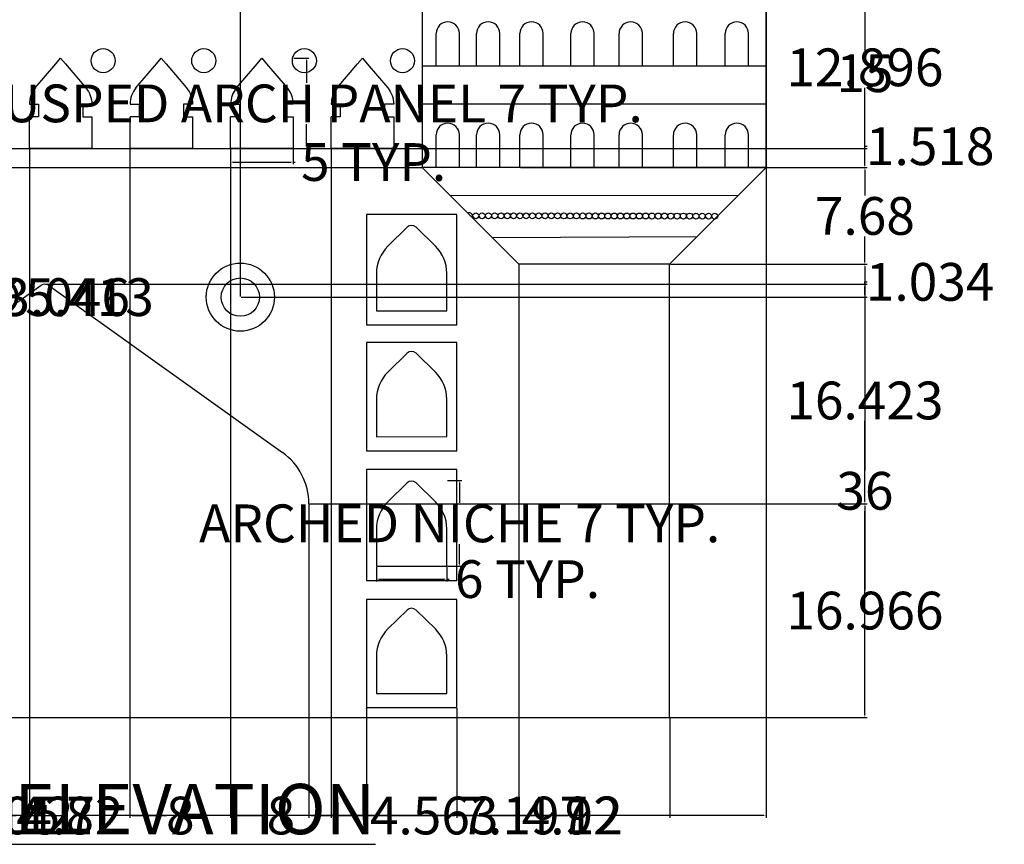
# Model space of a CAD drawing. Units: inches. Extents: x 168 to 318, y 152 to 314.
# Tile 5 of 7: x 240 to 318, y 152 to 218. Entities that reach past the tile are written whole.
import ezdxf

# ---------------------------------------------------------------- set-up
doc = ezdxf.new("R2010")
doc.units = ezdxf.units.IN
doc.header["$MEASUREMENT"] = 0
for name, color, linetype, lineweight in [('A-ANNO-DIMS', 2, 'Continuous', 18), ('A-ANNO-TEXT', 3, 'Continuous', 25), ('A-ELEV', 7, 'Continuous', 25)]:
    doc.layers.add(name, color=color, linetype=linetype, lineweight=lineweight)
doc.styles.get("Standard").update_dxf_attribs({"font": 'arial.ttf'})
doc.dimstyles.get("Standard").update_dxf_attribs({"dimtxt": 3, "dimasz": 0.18, "dimexe": 0.18, "dimexo": 0.0625, "dimgap": 0.09, "dimtad": 0, "dimtih": 1, "dimtoh": 1, "dimdec": 1, "dimzin": 0, "dimdsep": 46, "dimlunit": 3, "dimtxsty": 'Standard', "dimcen": 0.09, "dimadec": 0, "dimazin": 0, "dimtfac": 1, "dimtdec": 1, "dimtofl": 0, "dimtmove": 0, "dimatfit": 3, "dimfxl": 1, "dimtolj": 1, "dimtzin": 0, "dimarcsym": 0})

# ---------------------------------------------------------------- blocks, each defined once
blk = doc.blocks.new('ARCH-BALCONY-SM')
for p, q in [((0, 0), (0, 2.603)), ((1.853, 0), (1.853, 2.603))]:
    blk.add_line(p, q)
blk.add_arc((0.926, 2.603), 0.926, 0, 180)
blk = doc.blocks.new('ARCH-CUSPED-PANEL')
for p, q in [((2.1, 6.738), (2.482, 7.168)), ((2.482, 7.168), (2.864, 6.738)), ((0.472, 4.813), (2.1, 6.738)), ((2.864, 6.738), (4.491, 4.813)), ((0, 3.522), (0.2, 3.522)), ((0, 3.522), (0, 3.522)), ((0.2, 3.522), (0.719, 3.522)), ((0.719, 3.522), (0.719, 2.522)), ((4.764, 3.522), (4.244, 3.522)), ((4.244, 3.522), (4.244, 2.522)), ((4.964, 3.522), (4.764, 3.522)), ((0.719, 2.522), (0, 2.522)), ((4.244, 2.522), (4.964, 2.522))]:
    blk.add_line(p, q)
blk.add_lwpolyline([(4.491, 4.813, -0.177277), (4.964, 3.522)], format="xyb")
blk.add_lwpolyline([(4.964, 2.522), (4.964, 0), (0, 0), (0, 2.522)])
blk.add_arc((2, 3.522), 2, 139.78884, 180)
blk = doc.blocks.new('NICHE-ARCHED')
for p, q in [((0.908, 5.124), (2.451, 6.627)), ((3.149, 6.626), (4.687, 5.124)), ((0, 2.975), (0, 0)), ((5.592, 0), (5.592, 2.977)), ((0, 0), (5.592, 0))]:
    blk.add_line(p, q)
for centre, radius, start, end in [((2.8, 6.268), 0.5, 45.68441, 134.22565), ((3, 2.975), 3, 134.22565, 180), ((2.592, 2.977), 3, 0, 45.68441)]:
    blk.add_arc(centre, radius, start, end)
blk = doc.blocks.new('*D15')
at = {"layer": 'A-ANNO-DIMS', "color": 0, "lineweight": -2, "ltscale": 0.2, "transparency": 16777216}
for p, q in [((214.946, 220.875), (215.434, 220.875)), ((215.254, 220.875), (215.254, 221.055)), ((215.254, 221.055), (215.434, 221.055)), ((215.254, 218.586), (215.254, 220.695)), ((214.946, 218.406), (215.434, 218.406))]:
    blk.add_line(p, q, dxfattribs=at)
at = {"layer": 'A-ANNO-DIMS', "color": 0, "ltscale": 0.2, "transparency": 16777216}
for points in [[(215.224, 220.695), (215.284, 220.695), (215.254, 220.875)], [(215.224, 218.586), (215.284, 218.586), (215.254, 218.406)]]:
    blk.add_solid(points, dxfattribs=at)
at = {"layer": 'Defpoints', "color": 0, "ltscale": 0.2, "transparency": 16777216}
for p in [(214.883, 220.875), (215.254, 220.875), (214.883, 218.406)]:
    blk.add_point(p, dxfattribs=at)
at = {"layer": 'A-ANNO-DIMS', "color": 0, "ltscale": 0.2, "transparency": 16777216, "insert": (244.753, 221.055), "char_height": 3, "attachment_point": 5}
blk.add_mtext('\\A1;PENDANT ORNAMENT 2 TYP.', dxfattribs=at)
blk = doc.blocks.new('*D21')
at = {"layer": 'A-ANNO-DIMS', "color": 0, "lineweight": -2, "ltscale": 0.2, "transparency": 16777216}
for p, q in [((274.104, 181.018), (275.244, 181.018)), ((275.064, 180.838), (275.065, 179.251)), ((275.067, 174.382), (275.066, 175.969)), ((274.107, 174.202), (275.247, 174.202))]:
    blk.add_line(p, q, dxfattribs=at)
at = {"layer": 'A-ANNO-DIMS', "color": 0, "ltscale": 0.2, "transparency": 16777216}
for points in [[(275.094, 180.838), (275.034, 180.838), (275.064, 181.018)], [(275.097, 174.382), (275.037, 174.382), (275.067, 174.202)]]:
    blk.add_solid(points, dxfattribs=at)
at = {"layer": 'Defpoints', "color": 0, "ltscale": 0.2, "transparency": 16777216}
for p in [(274.041, 181.018), (275.064, 181.018), (274.045, 174.202)]:
    blk.add_point(p, dxfattribs=at)
at = {"layer": 'A-ANNO-DIMS', "color": 0, "ltscale": 0.2, "transparency": 16777216, "insert": (275.066, 177.61), "char_height": 3, "attachment_point": 5}
blk.add_mtext('\\A1;ARCHED NICHE 7 TYP.', dxfattribs=at)
blk = doc.blocks.new('*D22')
at = {"layer": 'A-ANNO-DIMS', "color": 0, "lineweight": -2, "ltscale": 0.2, "transparency": 16777216}
for p, q in [((268.453, 174.136), (268.454, 172.996)), ((274.045, 174.139), (274.045, 172.999)), ((268.634, 173.177), (273.865, 173.179)), ((274.045, 173.179), (274.225, 173.179))]:
    blk.add_line(p, q, dxfattribs=at)
at = {"layer": 'A-ANNO-DIMS', "color": 0, "ltscale": 0.2, "transparency": 16777216}
for points in [[(268.634, 173.207), (268.634, 173.147), (268.454, 173.176)], [(273.865, 173.209), (273.865, 173.149), (274.045, 173.179)]]:
    blk.add_solid(points, dxfattribs=at)
at = {"layer": 'Defpoints', "color": 0, "ltscale": 0.2, "transparency": 16777216}
for p in [(268.453, 174.199), (274.045, 174.202), (274.045, 173.179)]:
    blk.add_point(p, dxfattribs=at)
at = {"layer": 'A-ANNO-DIMS', "color": 0, "ltscale": 0.2, "transparency": 16777216, "insert": (280.46, 173.179), "char_height": 3, "attachment_point": 5}
blk.add_mtext('\\A1;6 TYP.', dxfattribs=at)
blk = doc.blocks.new('*D23')
at = {"layer": 'A-ANNO-DIMS', "color": 0, "lineweight": -2, "ltscale": 0.2, "transparency": 16777216}
for p, q in [((261.882, 214.562), (263.075, 214.562)), ((262.895, 214.382), (262.895, 212.619)), ((262.895, 207.574), (262.895, 209.337)), ((261.882, 207.394), (263.075, 207.394))]:
    blk.add_line(p, q, dxfattribs=at)
at = {"layer": 'A-ANNO-DIMS', "color": 0, "ltscale": 0.2, "transparency": 16777216}
for points in [[(262.865, 214.382), (262.925, 214.382), (262.895, 214.562)], [(262.865, 207.574), (262.925, 207.574), (262.895, 207.394)]]:
    blk.add_solid(points, dxfattribs=at)
at = {"layer": 'Defpoints', "color": 0, "ltscale": 0.2, "transparency": 16777216}
for p in [(261.82, 214.562), (262.895, 214.562), (261.82, 207.394)]:
    blk.add_point(p, dxfattribs=at)
at = {"layer": 'A-ANNO-DIMS', "color": 0, "ltscale": 0.2, "transparency": 16777216, "insert": (262.895, 210.978), "char_height": 3, "attachment_point": 5}
blk.add_mtext('\\A1;CUSPED ARCH PANEL 7 TYP.', dxfattribs=at)
blk = doc.blocks.new('*D24')
at = {"layer": 'A-ANNO-DIMS', "color": 0, "lineweight": -2, "ltscale": 0.2, "transparency": 16777216}
for p, q in [((256.855, 207.331), (256.855, 206.138)), ((261.82, 207.331), (261.82, 206.138)), ((257.035, 206.318), (261.64, 206.318)), ((261.82, 206.318), (262, 206.318))]:
    blk.add_line(p, q, dxfattribs=at)
at = {"layer": 'A-ANNO-DIMS', "color": 0, "ltscale": 0.2, "transparency": 16777216}
for points in [[(257.035, 206.348), (257.035, 206.288), (256.855, 206.318)], [(261.64, 206.348), (261.64, 206.288), (261.82, 206.318)]]:
    blk.add_solid(points, dxfattribs=at)
at = {"layer": 'Defpoints', "color": 0, "ltscale": 0.2, "transparency": 16777216}
for p in [(256.855, 207.394), (261.82, 207.394), (261.82, 206.318)]:
    blk.add_point(p, dxfattribs=at)
at = {"layer": 'A-ANNO-DIMS', "color": 0, "ltscale": 0.2, "transparency": 16777216, "insert": (268.226, 206.318), "char_height": 3, "attachment_point": 5}
blk.add_mtext('\\A1;5 TYP.', dxfattribs=at)
blk = doc.blocks.new('*D29')
at = {"layer": 'A-ANNO-DIMS', "color": 0, "lineweight": -2, "ltscale": 0.2, "transparency": 16777216}
for p, q in [((184.724, 242.139), (184.724, 154.215)), ((299.445, 242.139), (299.445, 154.215)), ((184.904, 154.395), (235.924, 154.395)), ((299.265, 154.395), (248.245, 154.395))]:
    blk.add_line(p, q, dxfattribs=at)
at = {"layer": 'A-ANNO-DIMS', "color": 0, "ltscale": 0.2, "transparency": 16777216}
for points in [[(184.904, 154.425), (184.904, 154.365), (184.724, 154.395)], [(299.265, 154.425), (299.265, 154.365), (299.445, 154.395)]]:
    blk.add_solid(points, dxfattribs=at)
at = {"layer": 'Defpoints', "color": 0, "ltscale": 0.2, "transparency": 16777216}
for p in [(184.724, 242.201), (299.445, 242.201), (299.445, 154.395)]:
    blk.add_point(p, dxfattribs=at)
at = {"layer": 'A-ANNO-DIMS', "color": 0, "ltscale": 0.2, "transparency": 16777216, "insert": (242.084, 154.395), "char_height": 3, "attachment_point": 5}
blk.add_mtext('\\A1;114.72', dxfattribs=at)
blk = doc.blocks.new('*D34')
at = {"layer": 'A-ANNO-DIMS', "color": 0, "lineweight": -2, "ltscale": 0.2, "transparency": 16777216}
for p, q in [((291.827, 198.195), (307.468, 198.195)), ((307.288, 198.015), (307.288, 181.818)), ((307.288, 162.375), (307.288, 178.573)), ((291.827, 162.195), (307.468, 162.195))]:
    blk.add_line(p, q, dxfattribs=at)
at = {"layer": 'A-ANNO-DIMS', "color": 0, "ltscale": 0.2, "transparency": 16777216}
for points in [[(307.258, 198.015), (307.318, 198.015), (307.288, 198.195)], [(307.258, 162.375), (307.318, 162.375), (307.288, 162.195)]]:
    blk.add_solid(points, dxfattribs=at)
at = {"layer": 'Defpoints', "color": 0, "ltscale": 0.2, "transparency": 16777216}
for p in [(291.765, 198.195), (307.288, 198.195), (291.765, 162.195)]:
    blk.add_point(p, dxfattribs=at)
at = {"layer": 'A-ANNO-DIMS', "color": 0, "ltscale": 0.2, "transparency": 16777216, "insert": (307.288, 180.195), "char_height": 3, "attachment_point": 5}
blk.add_mtext('\\A1;36', dxfattribs=at)
blk = doc.blocks.new('*D35')
at = {"layer": 'A-ANNO-DIMS', "color": 0, "lineweight": -2, "ltscale": 0.2, "transparency": 16777216}
for p, q in [((299.507, 205.875), (307.468, 205.875)), ((307.288, 205.695), (307.288, 203.657)), ((307.288, 198.375), (307.288, 200.414)), ((291.827, 198.195), (307.468, 198.195))]:
    blk.add_line(p, q, dxfattribs=at)
at = {"layer": 'A-ANNO-DIMS', "color": 0, "ltscale": 0.2, "transparency": 16777216}
for points in [[(307.258, 205.695), (307.318, 205.695), (307.288, 205.875)], [(307.258, 198.375), (307.318, 198.375), (307.288, 198.195)]]:
    blk.add_solid(points, dxfattribs=at)
at = {"layer": 'Defpoints', "color": 0, "ltscale": 0.2, "transparency": 16777216}
for p in [(299.445, 205.875), (307.288, 205.875), (291.765, 198.195)]:
    blk.add_point(p, dxfattribs=at)
at = {"layer": 'A-ANNO-DIMS', "color": 0, "ltscale": 0.2, "transparency": 16777216, "insert": (307.288, 202.035), "char_height": 3, "attachment_point": 5}
blk.add_mtext('\\A1;7.68', dxfattribs=at)
blk = doc.blocks.new('*D36')
at = {"layer": 'A-ANNO-DIMS', "color": 0, "lineweight": -2, "ltscale": 0.2, "transparency": 16777216}
for p, q in [((299.507, 220.875), (307.468, 220.875)), ((307.288, 220.695), (307.288, 214.997)), ((307.288, 206.055), (307.288, 211.754)), ((299.507, 205.875), (307.468, 205.875))]:
    blk.add_line(p, q, dxfattribs=at)
at = {"layer": 'A-ANNO-DIMS', "color": 0, "ltscale": 0.2, "transparency": 16777216}
for points in [[(307.258, 220.695), (307.318, 220.695), (307.288, 220.875)], [(307.258, 206.055), (307.318, 206.055), (307.288, 205.875)]]:
    blk.add_solid(points, dxfattribs=at)
at = {"layer": 'Defpoints', "color": 0, "ltscale": 0.2, "transparency": 16777216}
for p in [(299.445, 220.875), (307.288, 220.875), (299.445, 205.875)]:
    blk.add_point(p, dxfattribs=at)
at = {"layer": 'A-ANNO-DIMS', "color": 0, "ltscale": 0.2, "transparency": 16777216, "insert": (307.288, 213.375), "char_height": 3, "attachment_point": 5}
blk.add_mtext('\\A1;15', dxfattribs=at)
blk = doc.blocks.new('*D52')
at = {"layer": 'A-ANNO-DIMS', "color": 0, "lineweight": -2, "ltscale": 0.2, "transparency": 16777216}
for p, q in [((221.084, 162.133), (221.084, 154.215)), ((263.084, 162.133), (263.084, 154.215)), ((221.264, 154.395), (239.801, 154.395)), ((262.904, 154.395), (244.368, 154.395))]:
    blk.add_line(p, q, dxfattribs=at)
at = {"layer": 'A-ANNO-DIMS', "color": 0, "ltscale": 0.2, "transparency": 16777216}
for points in [[(221.264, 154.425), (221.264, 154.365), (221.084, 154.395)], [(262.904, 154.425), (262.904, 154.365), (263.084, 154.395)]]:
    blk.add_solid(points, dxfattribs=at)
at = {"layer": 'Defpoints', "color": 0, "ltscale": 0.2, "transparency": 16777216}
for p in [(221.084, 162.195), (263.084, 162.195), (263.084, 154.395)]:
    blk.add_point(p, dxfattribs=at)
at = {"layer": 'A-ANNO-DIMS', "color": 0, "ltscale": 0.2, "transparency": 16777216, "insert": (242.084, 154.395), "char_height": 3, "attachment_point": 5}
blk.add_mtext('\\A1;42', dxfattribs=at)
blk = doc.blocks.new('*D53')
at = {"layer": 'A-ANNO-DIMS', "color": 0, "lineweight": -2, "ltscale": 0.2, "transparency": 16777216}
for p, q in [((267.647, 162.916), (267.647, 154.215)), ((263.084, 162.133), (263.084, 154.215)), ((263.264, 154.395), (267.467, 154.395)), ((267.647, 154.395), (267.827, 154.395))]:
    blk.add_line(p, q, dxfattribs=at)
at = {"layer": 'A-ANNO-DIMS', "color": 0, "ltscale": 0.2, "transparency": 16777216}
for points in [[(263.264, 154.425), (263.264, 154.365), (263.084, 154.395)], [(267.467, 154.425), (267.467, 154.365), (267.647, 154.395)]]:
    blk.add_solid(points, dxfattribs=at)
at = {"layer": 'Defpoints', "color": 0, "ltscale": 0.2, "transparency": 16777216}
for p in [(267.647, 162.979), (263.084, 162.195), (267.647, 154.395)]:
    blk.add_point(p, dxfattribs=at)
at = {"layer": 'A-ANNO-DIMS', "color": 0, "ltscale": 0.2, "transparency": 16777216, "insert": (273.039, 154.395), "char_height": 3, "attachment_point": 5}
blk.add_mtext('\\A1;4.563', dxfattribs=at)
blk = doc.blocks.new('*D54')
at = {"layer": 'A-ANNO-DIMS', "color": 0, "lineweight": -2, "ltscale": 0.2, "transparency": 16777216}
for p, q in [((267.647, 162.916), (267.647, 154.215)), ((274.844, 162.916), (274.844, 154.215)), ((267.827, 154.395), (274.664, 154.395)), ((274.844, 154.395), (275.024, 154.395))]:
    blk.add_line(p, q, dxfattribs=at)
at = {"layer": 'A-ANNO-DIMS', "color": 0, "ltscale": 0.2, "transparency": 16777216}
for points in [[(267.827, 154.425), (267.827, 154.365), (267.647, 154.395)], [(274.664, 154.425), (274.664, 154.365), (274.844, 154.395)]]:
    blk.add_solid(points, dxfattribs=at)
at = {"layer": 'Defpoints', "color": 0, "ltscale": 0.2, "transparency": 16777216}
for p in [(267.647, 162.979), (274.844, 162.979), (274.844, 154.395)]:
    blk.add_point(p, dxfattribs=at)
at = {"layer": 'A-ANNO-DIMS', "color": 0, "ltscale": 0.2, "transparency": 16777216, "insert": (280.164, 154.395), "char_height": 3, "attachment_point": 5}
blk.add_mtext('\\A1;7.197', dxfattribs=at)
blk = doc.blocks.new('*D55')
at = {"layer": 'A-ANNO-DIMS', "color": 0, "lineweight": -2, "ltscale": 0.2, "transparency": 16777216}
for p, q in [((274.844, 162.916), (274.844, 154.215)), ((279.765, 162.133), (279.765, 154.215)), ((275.024, 154.395), (279.585, 154.395)), ((279.765, 154.395), (279.945, 154.395))]:
    blk.add_line(p, q, dxfattribs=at)
at = {"layer": 'A-ANNO-DIMS', "color": 0, "ltscale": 0.2, "transparency": 16777216}
for points in [[(275.024, 154.425), (275.024, 154.365), (274.844, 154.395)], [(279.585, 154.425), (279.585, 154.365), (279.765, 154.395)]]:
    blk.add_solid(points, dxfattribs=at)
at = {"layer": 'Defpoints', "color": 0, "ltscale": 0.2, "transparency": 16777216}
for p in [(274.844, 162.979), (279.765, 162.195), (279.765, 154.395)]:
    blk.add_point(p, dxfattribs=at)
at = {"layer": 'A-ANNO-DIMS', "color": 0, "ltscale": 0.2, "transparency": 16777216, "insert": (283.976, 154.395), "char_height": 3, "attachment_point": 5}
blk.add_mtext('\\A1;4.92', dxfattribs=at)
blk = doc.blocks.new('*D56')
at = {"layer": 'A-ANNO-DIMS', "color": 0, "lineweight": -2, "ltscale": 0.2, "transparency": 16777216}
for p, q in [((279.765, 162.133), (279.765, 154.215)), ((291.765, 162.133), (291.765, 154.215)), ((279.945, 154.395), (283.682, 154.395)), ((291.585, 154.395), (287.847, 154.395))]:
    blk.add_line(p, q, dxfattribs=at)
at = {"layer": 'A-ANNO-DIMS', "color": 0, "ltscale": 0.2, "transparency": 16777216}
for points in [[(279.945, 154.425), (279.945, 154.365), (279.765, 154.395)], [(291.585, 154.425), (291.585, 154.365), (291.765, 154.395)]]:
    blk.add_solid(points, dxfattribs=at)
at = {"layer": 'Defpoints', "color": 0, "ltscale": 0.2, "transparency": 16777216}
for p in [(279.765, 162.195), (291.765, 162.195), (291.765, 154.395)]:
    blk.add_point(p, dxfattribs=at)
at = {"layer": 'A-ANNO-DIMS', "color": 0, "ltscale": 0.2, "transparency": 16777216, "insert": (285.765, 154.395), "char_height": 3, "attachment_point": 5}
blk.add_mtext('\\A1;12', dxfattribs=at)
blk = doc.blocks.new('*D57')
at = {"layer": 'A-ANNO-DIMS', "color": 0, "lineweight": -2, "ltscale": 0.2, "transparency": 16777216}
for p, q in [((226.54, 195.647), (226.54, 312.411)), ((257.629, 195.647), (257.629, 312.411)), ((226.72, 312.231), (236.931, 312.231)), ((257.449, 312.231), (247.238, 312.231))]:
    blk.add_line(p, q, dxfattribs=at)
at = {"layer": 'A-ANNO-DIMS', "color": 0, "ltscale": 0.2, "transparency": 16777216}
for points in [[(226.72, 312.261), (226.72, 312.201), (226.54, 312.231)], [(257.449, 312.261), (257.449, 312.201), (257.629, 312.231)]]:
    blk.add_solid(points, dxfattribs=at)
at = {"layer": 'Defpoints', "color": 0, "ltscale": 0.2, "transparency": 16777216}
for p in [(257.629, 312.231), (226.54, 195.584), (257.629, 195.584)]:
    blk.add_point(p, dxfattribs=at)
at = {"layer": 'A-ANNO-DIMS', "color": 0, "ltscale": 0.2, "transparency": 16777216, "insert": (242.084, 312.231), "char_height": 3, "attachment_point": 5}
blk.add_mtext('\\A1;31.09', dxfattribs=at)
blk = doc.blocks.new('*D63')
at = {"layer": 'A-ANNO-DIMS', "color": 0, "lineweight": -2, "ltscale": 0.2, "transparency": 16777216}
for p, q in [((263.147, 179.161), (307.468, 179.161)), ((307.288, 178.981), (307.288, 172.3)), ((307.288, 162.375), (307.288, 169.057)), ((263.147, 162.195), (307.468, 162.195))]:
    blk.add_line(p, q, dxfattribs=at)
at = {"layer": 'A-ANNO-DIMS', "color": 0, "ltscale": 0.2, "transparency": 16777216}
for points in [[(307.258, 178.981), (307.318, 178.981), (307.288, 179.161)], [(307.258, 162.375), (307.318, 162.375), (307.288, 162.195)]]:
    blk.add_solid(points, dxfattribs=at)
at = {"layer": 'Defpoints', "color": 0, "ltscale": 0.2, "transparency": 16777216}
for p in [(263.084, 179.161), (307.288, 179.161), (263.084, 162.195)]:
    blk.add_point(p, dxfattribs=at)
at = {"layer": 'A-ANNO-DIMS', "color": 0, "ltscale": 0.2, "transparency": 16777216, "insert": (307.288, 170.678), "char_height": 3, "attachment_point": 5}
blk.add_mtext('\\A1;16.966', dxfattribs=at)
blk = doc.blocks.new('*D64')
at = {"layer": 'A-ANNO-DIMS', "color": 0, "lineweight": -2, "ltscale": 0.2, "transparency": 16777216}
for p, q in [((257.691, 195.584), (307.468, 195.584)), ((307.288, 195.404), (307.288, 188.996)), ((307.288, 179.341), (307.288, 185.75)), ((263.147, 179.161), (307.468, 179.161))]:
    blk.add_line(p, q, dxfattribs=at)
at = {"layer": 'A-ANNO-DIMS', "color": 0, "ltscale": 0.2, "transparency": 16777216}
for points in [[(307.258, 195.404), (307.318, 195.404), (307.288, 195.584)], [(307.258, 179.341), (307.318, 179.341), (307.288, 179.161)]]:
    blk.add_solid(points, dxfattribs=at)
at = {"layer": 'Defpoints', "color": 0, "ltscale": 0.2, "transparency": 16777216}
for p in [(257.629, 195.584), (307.288, 195.584), (263.084, 179.161)]:
    blk.add_point(p, dxfattribs=at)
at = {"layer": 'A-ANNO-DIMS', "color": 0, "ltscale": 0.2, "transparency": 16777216, "insert": (307.288, 187.373), "char_height": 3, "attachment_point": 5}
blk.add_mtext('\\A1;16.423', dxfattribs=at)
blk = doc.blocks.new('*D65')
at = {"layer": 'A-ANNO-DIMS', "color": 0, "lineweight": -2, "ltscale": 0.2, "transparency": 16777216}
for p, q in [((242.147, 196.618), (307.468, 196.618)), ((307.288, 196.618), (307.288, 196.798)), ((307.288, 196.798), (307.468, 196.798)), ((307.288, 195.764), (307.288, 196.438)), ((257.691, 195.584), (307.468, 195.584))]:
    blk.add_line(p, q, dxfattribs=at)
at = {"layer": 'A-ANNO-DIMS', "color": 0, "ltscale": 0.2, "transparency": 16777216}
for points in [[(307.258, 196.438), (307.318, 196.438), (307.288, 196.618)], [(307.258, 195.764), (307.318, 195.764), (307.288, 195.584)]]:
    blk.add_solid(points, dxfattribs=at)
at = {"layer": 'Defpoints', "color": 0, "ltscale": 0.2, "transparency": 16777216}
for p in [(242.084, 196.618), (307.288, 196.618), (257.629, 195.584)]:
    blk.add_point(p, dxfattribs=at)
at = {"layer": 'A-ANNO-DIMS', "color": 0, "ltscale": 0.2, "transparency": 16777216, "insert": (312.473, 196.798), "char_height": 3, "attachment_point": 5}
blk.add_mtext('\\A1;1.034', dxfattribs=at)
blk = doc.blocks.new('*D75')
at = {"layer": 'A-ANNO-DIMS', "color": 0, "lineweight": -2, "ltscale": 0.2, "transparency": 16777216}
for p, q in [((307.288, 207.394), (307.288, 207.574)), ((307.288, 207.574), (307.468, 207.574)), ((272.147, 207.394), (307.468, 207.394)), ((307.288, 206.055), (307.288, 207.214)), ((279.916, 205.875), (307.468, 205.875))]:
    blk.add_line(p, q, dxfattribs=at)
at = {"layer": 'A-ANNO-DIMS', "color": 0, "ltscale": 0.2, "transparency": 16777216}
for points in [[(307.258, 207.214), (307.318, 207.214), (307.288, 207.394)], [(307.258, 206.055), (307.318, 206.055), (307.288, 205.875)]]:
    blk.add_solid(points, dxfattribs=at)
at = {"layer": 'Defpoints', "color": 0, "ltscale": 0.2, "transparency": 16777216}
for p in [(272.084, 207.394), (307.288, 207.394), (279.854, 205.875)]:
    blk.add_point(p, dxfattribs=at)
at = {"layer": 'A-ANNO-DIMS', "color": 0, "ltscale": 0.2, "transparency": 16777216, "insert": (312.482, 207.574), "char_height": 3, "attachment_point": 5}
blk.add_mtext('\\A1;1.518', dxfattribs=at)
blk = doc.blocks.new('*D76')
at = {"layer": 'A-ANNO-DIMS', "color": 0, "lineweight": -2, "ltscale": 0.2, "transparency": 16777216}
for p, q in [((279.689, 220.29), (307.468, 220.29)), ((307.288, 220.11), (307.288, 215.463)), ((307.288, 207.574), (307.288, 212.22)), ((272.147, 207.394), (307.468, 207.394))]:
    blk.add_line(p, q, dxfattribs=at)
at = {"layer": 'A-ANNO-DIMS', "color": 0, "ltscale": 0.2, "transparency": 16777216}
for points in [[(307.258, 220.11), (307.318, 220.11), (307.288, 220.29)], [(307.258, 207.574), (307.318, 207.574), (307.288, 207.394)]]:
    blk.add_solid(points, dxfattribs=at)
at = {"layer": 'Defpoints', "color": 0, "ltscale": 0.2, "transparency": 16777216}
for p in [(279.627, 220.29), (307.288, 220.29), (272.084, 207.394)]:
    blk.add_point(p, dxfattribs=at)
at = {"layer": 'A-ANNO-DIMS', "color": 0, "ltscale": 0.2, "transparency": 16777216, "insert": (307.288, 213.842), "char_height": 3, "attachment_point": 5}
blk.add_mtext('\\A1;12.896', dxfattribs=at)
blk = doc.blocks.new('*D90')
at = {"layer": 'A-ANNO-DIMS', "color": 0, "lineweight": -2, "ltscale": 0.2, "transparency": 16777216}
for p, q in [((224.151, 207.331), (224.151, 154.215)), ((232.855, 207.331), (232.855, 154.215)), ((224.331, 154.395), (232.675, 154.395)), ((232.855, 154.395), (233.035, 154.395))]:
    blk.add_line(p, q, dxfattribs=at)
at = {"layer": 'A-ANNO-DIMS', "color": 0, "ltscale": 0.2, "transparency": 16777216}
for points in [[(224.331, 154.425), (224.331, 154.365), (224.151, 154.395)], [(232.675, 154.425), (232.675, 154.365), (232.855, 154.395)]]:
    blk.add_solid(points, dxfattribs=at)
at = {"layer": 'Defpoints', "color": 0, "ltscale": 0.2, "transparency": 16777216}
for p in [(224.151, 207.394), (232.855, 207.394), (232.855, 154.395)]:
    blk.add_point(p, dxfattribs=at)
at = {"layer": 'A-ANNO-DIMS', "color": 0, "ltscale": 0.2, "transparency": 16777216, "insert": (238.2, 154.395), "char_height": 3, "attachment_point": 5}
blk.add_mtext('\\A1;8.705', dxfattribs=at)
blk = doc.blocks.new('*D91')
at = {"layer": 'A-ANNO-DIMS', "color": 0, "lineweight": -2, "ltscale": 0.2, "transparency": 16777216}
for p, q in [((232.855, 207.331), (232.855, 154.215)), ((240.855, 207.331), (240.855, 154.215)), ((233.035, 154.395), (235.777, 154.395)), ((240.675, 154.395), (237.934, 154.395))]:
    blk.add_line(p, q, dxfattribs=at)
at = {"layer": 'A-ANNO-DIMS', "color": 0, "ltscale": 0.2, "transparency": 16777216}
for points in [[(233.035, 154.425), (233.035, 154.365), (232.855, 154.395)], [(240.675, 154.425), (240.675, 154.365), (240.855, 154.395)]]:
    blk.add_solid(points, dxfattribs=at)
at = {"layer": 'Defpoints', "color": 0, "ltscale": 0.2, "transparency": 16777216}
for p in [(232.855, 207.394), (240.855, 207.394), (240.855, 154.395)]:
    blk.add_point(p, dxfattribs=at)
at = {"layer": 'A-ANNO-DIMS', "color": 0, "ltscale": 0.2, "transparency": 16777216, "insert": (236.855, 154.395), "char_height": 3, "attachment_point": 5}
blk.add_mtext('\\A1;8', dxfattribs=at)
blk = doc.blocks.new('*D92')
at = {"layer": 'A-ANNO-DIMS', "color": 0, "lineweight": -2, "ltscale": 0.2, "transparency": 16777216}
for p, q in [((240.855, 207.331), (240.855, 154.215)), ((248.855, 207.331), (248.855, 154.215)), ((241.035, 154.395), (243.777, 154.395)), ((248.675, 154.395), (245.934, 154.395))]:
    blk.add_line(p, q, dxfattribs=at)
at = {"layer": 'A-ANNO-DIMS', "color": 0, "ltscale": 0.2, "transparency": 16777216}
for points in [[(241.035, 154.425), (241.035, 154.365), (240.855, 154.395)], [(248.675, 154.425), (248.675, 154.365), (248.855, 154.395)]]:
    blk.add_solid(points, dxfattribs=at)
at = {"layer": 'Defpoints', "color": 0, "ltscale": 0.2, "transparency": 16777216}
for p in [(240.855, 207.394), (248.855, 207.394), (248.855, 154.395)]:
    blk.add_point(p, dxfattribs=at)
at = {"layer": 'A-ANNO-DIMS', "color": 0, "ltscale": 0.2, "transparency": 16777216, "insert": (244.855, 154.395), "char_height": 3, "attachment_point": 5}
blk.add_mtext('\\A1;8', dxfattribs=at)
blk = doc.blocks.new('*D93')
at = {"layer": 'A-ANNO-DIMS', "color": 0, "lineweight": -2, "ltscale": 0.2, "transparency": 16777216}
for p, q in [((248.855, 207.331), (248.855, 154.215)), ((256.855, 207.331), (256.855, 154.215)), ((249.035, 154.395), (251.777, 154.395)), ((256.675, 154.395), (253.934, 154.395))]:
    blk.add_line(p, q, dxfattribs=at)
at = {"layer": 'A-ANNO-DIMS', "color": 0, "ltscale": 0.2, "transparency": 16777216}
for points in [[(249.035, 154.425), (249.035, 154.365), (248.855, 154.395)], [(256.675, 154.425), (256.675, 154.365), (256.855, 154.395)]]:
    blk.add_solid(points, dxfattribs=at)
at = {"layer": 'Defpoints', "color": 0, "ltscale": 0.2, "transparency": 16777216}
for p in [(248.855, 207.394), (256.855, 207.394), (256.855, 154.395)]:
    blk.add_point(p, dxfattribs=at)
at = {"layer": 'A-ANNO-DIMS', "color": 0, "ltscale": 0.2, "transparency": 16777216, "insert": (252.855, 154.395), "char_height": 3, "attachment_point": 5}
blk.add_mtext('\\A1;8', dxfattribs=at)
blk = doc.blocks.new('*D94')
at = {"layer": 'A-ANNO-DIMS', "color": 0, "lineweight": -2, "ltscale": 0.2, "transparency": 16777216}
for p, q in [((256.855, 207.331), (256.855, 154.215)), ((264.855, 207.331), (264.855, 154.215)), ((257.035, 154.395), (259.777, 154.395)), ((264.675, 154.395), (261.934, 154.395))]:
    blk.add_line(p, q, dxfattribs=at)
at = {"layer": 'A-ANNO-DIMS', "color": 0, "ltscale": 0.2, "transparency": 16777216}
for points in [[(257.035, 154.425), (257.035, 154.365), (256.855, 154.395)], [(264.675, 154.425), (264.675, 154.365), (264.855, 154.395)]]:
    blk.add_solid(points, dxfattribs=at)
at = {"layer": 'Defpoints', "color": 0, "ltscale": 0.2, "transparency": 16777216}
for p in [(256.855, 207.394), (264.855, 207.394), (264.855, 154.395)]:
    blk.add_point(p, dxfattribs=at)
at = {"layer": 'A-ANNO-DIMS', "color": 0, "ltscale": 0.2, "transparency": 16777216, "insert": (260.855, 154.395), "char_height": 3, "attachment_point": 5}
blk.add_mtext('\\A1;8', dxfattribs=at)
blk = doc.blocks.new('*D98')
at = {"layer": 'A-ANNO-DIMS', "color": 0, "lineweight": -2, "ltscale": 0.2, "transparency": 16777216}
for p, q in [((226.45, 195.584), (226.63, 195.584)), ((226.54, 195.494), (226.54, 195.674)), ((230.871, 195.584), (229.427, 195.584))]:
    blk.add_line(p, q, dxfattribs=at)
at = {"layer": 'A-ANNO-DIMS', "color": 0, "ltscale": 0.2, "transparency": 16777216}
blk.add_solid([(229.427, 195.614), (229.427, 195.554), (229.247, 195.584)], dxfattribs=at)
at = {"layer": 'Defpoints', "color": 0, "ltscale": 0.2, "transparency": 16777216}
for p in [(223.834, 195.585), (229.247, 195.584)]:
    blk.add_point(p, dxfattribs=at)
at = {"layer": 'A-ANNO-DIMS', "color": 0, "ltscale": 0.2, "transparency": 16777216, "insert": (240.824, 195.584), "char_height": 3, "attachment_point": 5}
blk.add_mtext('\\A1;2X ∅5.413', dxfattribs=at)
blk = doc.blocks.new('*D99')
at = {"layer": 'A-ANNO-DIMS', "color": 0, "lineweight": -2, "ltscale": 0.2, "transparency": 16777216}
for p, q in [((226.45, 195.584), (226.63, 195.584)), ((226.54, 195.494), (226.54, 195.674)), ((228.977, 195.584), (228.243, 195.584))]:
    blk.add_line(p, q, dxfattribs=at)
at = {"layer": 'A-ANNO-DIMS', "color": 0, "ltscale": 0.2, "transparency": 16777216}
blk.add_solid([(228.243, 195.614), (228.243, 195.554), (228.063, 195.584)], dxfattribs=at)
at = {"layer": 'Defpoints', "color": 0, "ltscale": 0.2, "transparency": 16777216}
for p in [(225.017, 195.585), (228.063, 195.584)]:
    blk.add_point(p, dxfattribs=at)
at = {"layer": 'A-ANNO-DIMS', "color": 0, "ltscale": 0.2, "transparency": 16777216, "insert": (238.928, 195.584), "char_height": 3, "attachment_point": 5}
blk.add_mtext('\\A1;2X ∅3.046', dxfattribs=at)

msp = doc.modelspace()

# ---------------------------------------------------------------- linework, layer by layer
at = {"layer": 'A-ELEV'}
for p, q in [((272.0845, 220.8755), (272.0845, 205.8755)), ((299.4446, 205.8755), (299.4446, 220.8755)), ((299.4446, 213.9241), (272.0845, 213.9241)), ((299.4446, 210.9241), (272.0845, 210.9241)), ((212.0845, 207.3935), (272.0845, 207.3935)), ((299.4446, 205.8755), (272.0845, 205.8755)), ((279.7645, 198.1954), (272.0845, 205.8755)), ((291.7645, 198.1954), (299.4446, 205.8755)), ((297.2168, 203.6477), (274.3285, 203.6314)), ((293.9532, 200.3841), (277.6579, 200.302)), ((291.7645, 198.1954), (279.7645, 198.1954)), ((279.7645, 198.1954), (279.7645, 162.1954)), ((291.7645, 162.1954), (291.7645, 198.1954)), ((239.1785, 194.6573), (241.7939, 196.5252)), ((242.3751, 196.5252), (244.9905, 194.6573)), ((244.9905, 194.6573), (260.9905, 183.2299)), ((263.0845, 179.1611), (263.0845, 171.0451)), ((263.0845, 171.0451), (263.0845, 162.1954)), ((204.4044, 162.1954), (279.7645, 162.1954)), ((279.7645, 162.1954), (291.7645, 162.1954))]:
    msp.add_line(p, q, dxfattribs=at)
at = {"layer": 'A-ELEV', "ltscale": 0.2}
msp.add_line((212.0845, 205.8755), (272.0845, 205.8755), dxfattribs=at)
at = {"layer": 'A-ELEV'}
for points in [[(274.8441, 202.1566), (267.6473, 202.1566), (267.6473, 193.3878), (274.8441, 193.3878)], [(274.8441, 191.9874), (267.6473, 191.9874), (267.6473, 183.3788), (274.8441, 183.3788)], [(274.8441, 181.9003), (267.6473, 181.9003), (267.6473, 173.0824), (274.8441, 173.0824)], [(274.8441, 171.5491), (267.6473, 171.5491), (267.6473, 162.9789), (274.8441, 162.9789)]]:
    msp.add_lwpolyline(points, close=True, dxfattribs=at)
for centre, radius in [((246.7185, 214.3715), 0.9548), ((254.7185, 214.3715), 0.9548), ((262.7185, 214.3715), 0.9548), ((270.5185, 214.3715), 0.9548), ((276.354, 202.0476), 0.2354), ((276.854, 202.0469), 0.2354), ((277.354, 202.0462), 0.2354), ((277.854, 202.0455), 0.2354), ((278.354, 202.0447), 0.2354), ((278.854, 202.044), 0.2354), ((279.354, 202.0433), 0.2354), ((279.854, 202.0426), 0.2354), ((280.354, 202.0419), 0.2354), ((280.854, 202.0412), 0.2354), ((281.354, 202.0404), 0.2354), ((281.854, 202.0397), 0.2354), ((282.354, 202.039), 0.2354), ((282.854, 202.0383), 0.2354), ((283.354, 202.0376), 0.2354), ((283.854, 202.0369), 0.2354), ((284.354, 202.0361), 0.2354), ((284.854, 202.0354), 0.2354), ((285.354, 202.0347), 0.2354), ((285.854, 202.034), 0.2354), ((286.354, 202.0333), 0.2354), ((286.854, 202.0326), 0.2354), ((287.354, 202.0318), 0.2354), ((287.854, 202.0311), 0.2354), ((288.354, 202.0304), 0.2354), ((288.854, 202.0297), 0.2354), ((289.354, 202.029), 0.2354), ((289.854, 202.0283), 0.2354), ((290.354, 202.0275), 0.2354), ((290.854, 202.0268), 0.2354), ((291.354, 202.0261), 0.2354), ((291.854, 202.0254), 0.2354), ((292.354, 202.0247), 0.2354), ((292.854, 202.024), 0.2354), ((293.354, 202.0232), 0.2354), ((293.854, 202.0225), 0.2354), ((294.354, 202.0218), 0.2354), ((294.854, 202.0211), 0.2354), ((295.354, 202.0204), 0.2354), ((257.6286, 195.5844), 2.7067), ((257.6286, 195.5844), 1.5229)]:
    msp.add_circle(centre, radius, dxfattribs=at)
for centre, radius, start, end in [((275.854, 202.0483), 0.2354, 324.95912, 125.04088), ((275.854, 202.0483), 0.2354, 324.95912, 125.04088), ((242.0845, 196.1183), 0.5, 54.465226, 125.534774), ((242.0845, 196.1183), 0.5, 54.465226, 125.534774), ((258.0845, 179.1611), 5, 0, 54.465226)]:
    msp.add_arc(centre, radius, start, end, dxfattribs=at)

# ---------------------------------------------------------------- block references
for name, p in [('ARCH-BALCONY-SM', (273.1935, 213.9237)), ('ARCH-BALCONY-SM', (276.4067, 213.9237)), ('ARCH-BALCONY-SM', (279.8536, 213.9237)), ('ARCH-BALCONY-SM', (283.9118, 213.9237)), ('ARCH-BALCONY-SM', (287.7406, 213.9237)), ('ARCH-BALCONY-SM', (292.0638, 213.9237)), ('ARCH-BALCONY-SM', (296.1823, 213.9237)), ('ARCH-CUSPED-PANEL', (240.8558, 207.394)), ('ARCH-CUSPED-PANEL', (248.8558, 207.394)), ('ARCH-CUSPED-PANEL', (256.8558, 207.394)), ('ARCH-CUSPED-PANEL', (264.8558, 207.394)), ('ARCH-BALCONY-SM', (273.1935, 205.875)), ('ARCH-BALCONY-SM', (276.4067, 205.875)), ('ARCH-BALCONY-SM', (279.8536, 205.875)), ('ARCH-BALCONY-SM', (283.9118, 205.875)), ('ARCH-BALCONY-SM', (287.7406, 205.875)), ('ARCH-BALCONY-SM', (292.0638, 205.875)), ('ARCH-BALCONY-SM', (296.1823, 205.875))]:
    msp.add_blockref(name, p, dxfattribs=at)
at = {"layer": 'A-ELEV', "rotation": 0.0280033483739919}
for p in [(268.4533, 194.5045), (268.4533, 184.4955), (268.4533, 174.1991), (268.4533, 164.0956)]:
    msp.add_blockref('NICHE-ARCHED', p, dxfattribs=at)

# ---------------------------------------------------------------- texts
at = {"layer": 'A-ANNO-TEXT', "ltscale": 0.2, "insert": (207.4369, 156.91), "char_height": 4, "attachment_point": 1}
msp.add_mtext_dynamic_manual_height_columns('{\\fArial|b1|i0|c0|p34;\\LCHARMINAR ELEVATION }', width=92.221498, gutter_width=1, heights=[0], dxfattribs=at)

# ---------------------------------------------------------------- dimensions: what is measured, and where the dimension line sits
at = {"layer": 'A-ANNO-DIMS', "ltscale": 0.2}
for base, p1, p2, override, picture, middle in [((257.6286, 312.2308), (226.5403, 195.5844), (257.6286, 195.5844), {"dimdec": 2, "dimlfac": 1, "dimrnd": 0, "dimzin": 0, "dimdsep": 46, "dimlunit": 2}, '*D57', (242.0845, 312.2308)), ((299.4446, 154.3954), (184.7244, 242.2013), (299.4446, 242.2013), {"dimdec": 2, "dimlfac": 1, "dimrnd": 0, "dimzin": 0, "dimdsep": 46, "dimlunit": 2}, '*D29', (242.0845, 154.3954)), ((232.8554, 154.3954), (224.1506, 207.3935), (232.8554, 207.3935), {"dimdec": 3, "dimlfac": 1, "dimrnd": 0, "dimzin": 0, "dimdsep": 46, "dimlunit": 2}, '*D90', (238.2004, 154.3954)), ((240.8554, 154.3954), (232.8554, 207.3935), (240.8554, 207.3935), {"dimdec": 0, "dimlfac": 1, "dimrnd": 0, "dimzin": 0, "dimdsep": 46, "dimlunit": 2}, '*D91', (236.8554, 154.3954)), ((248.8554, 154.3954), (240.8554, 207.3935), (248.8554, 207.3935), {"dimdec": 0, "dimlfac": 1, "dimrnd": 0, "dimzin": 0, "dimdsep": 46, "dimlunit": 2}, '*D92', (244.8554, 154.3954)), ((256.8554, 154.3954), (248.8554, 207.3935), (256.8554, 207.3935), {"dimdec": 0, "dimlfac": 1, "dimrnd": 0, "dimzin": 0, "dimdsep": 46, "dimlunit": 2}, '*D93', (252.8554, 154.3954)), ((264.8554, 154.3954), (256.8554, 207.3935), (264.8554, 207.3935), {"dimdec": 0, "dimlfac": 1, "dimrnd": 0, "dimzin": 0, "dimdsep": 46, "dimlunit": 2}, '*D94', (260.8554, 154.3954)), ((267.6473, 154.3954), (263.0845, 162.1954), (267.6473, 162.9789), {"dimdec": 3, "dimlfac": 1, "dimrnd": 0, "dimzin": 0, "dimdsep": 46, "dimlunit": 2}, '*D53', (273.0394, 154.3954)), ((274.8441, 154.3954), (267.6473, 162.9789), (274.8441, 162.9789), {"dimdec": 3, "dimlfac": 1, "dimrnd": 0, "dimzin": 0, "dimdsep": 46, "dimlunit": 2}, '*D54', (280.1636, 154.3954)), ((279.7645, 154.3954), (274.8441, 162.9789), (279.7645, 162.1954), {"dimdec": 2, "dimlfac": 1, "dimrnd": 0, "dimzin": 0, "dimdsep": 46, "dimlunit": 2}, '*D55', (283.9759, 154.3954)), ((263.0845, 154.3954), (221.0845, 162.1954), (263.0845, 162.1954), {"dimdec": 0, "dimlfac": 1, "dimrnd": 0, "dimzin": 0, "dimdsep": 46, "dimlunit": 2}, '*D52', (242.0845, 154.3954)), ((291.7645, 154.3954), (279.7645, 162.1954), (291.7645, 162.1954), {"dimdec": 0, "dimlfac": 1, "dimrnd": 0, "dimzin": 0, "dimdsep": 46, "dimlunit": 2}, '*D56', (285.7645, 154.3954))]:
    dim = msp.add_linear_dim(base=base, p1=p1, p2=p2, dimstyle='Standard', override=override, dxfattribs=at)
    dim.commit()
    dim.dimension.update_dxf_attribs({"geometry": picture, "text_midpoint": middle})
for base, p1, p2, angle, text, picture, middle in [((215.2539, 220.8755), (214.8834, 218.4056), (214.8834, 220.8755), 90, 'PENDANT ORNAMENT <> TYP.', '*D15', (244.7534, 221.0555)), ((262.8949, 214.5622), (261.8196, 207.3935), (261.8196, 214.5622), 90, 'CUSPED ARCH PANEL <> TYP.', '*D23', (262.8949, 210.9778)), ((275.0639, 181.0181), (274.0448, 174.2016), (274.0415, 181.0176), 90.028003, 'ARCHED NICHE <> TYP.', '*D21', (275.0655, 177.6101)), ((274.0453, 173.1792), (268.4534, 174.1989), (274.0448, 174.2016), 0.028003, '<> TYP.', '*D22', (280.4596, 173.1793))]:
    dim = msp.add_linear_dim(base=base, p1=p1, p2=p2, angle=angle, text=text, dimstyle='Standard', override={"dimdec": 0, "dimrnd": 0, "dimzin": 0, "dimlunit": 2}, dxfattribs=at)
    dim.commit()
    dim.dimension.update_dxf_attribs({"geometry": picture, "text_midpoint": middle})
for base, p1, p2, override, picture, middle in [((307.2884, 220.8755), (299.4446, 205.8755), (299.4446, 220.8755), {"dimdec": 0, "dimlfac": 1, "dimrnd": 0, "dimzin": 0, "dimdsep": 46, "dimlunit": 2}, '*D36', (307.2884, 213.3755)), ((307.2884, 220.2897), (272.0845, 207.3935), (279.6267, 220.2897), {"dimdec": 3, "dimlfac": 1, "dimrnd": 0, "dimzin": 0, "dimdsep": 46, "dimlunit": 2}, '*D76', (307.2884, 213.8416)), ((307.2884, 207.3935), (279.8535, 205.8755), (272.0845, 207.3935), {"dimdec": 3, "dimlfac": 1, "dimrnd": 0, "dimzin": 0, "dimdsep": 46, "dimlunit": 2}, '*D75', (312.482, 207.5735)), ((307.2884, 205.8755), (291.7645, 198.1954), (299.4446, 205.8755), {"dimdec": 2, "dimlfac": 1, "dimrnd": 0, "dimzin": 0, "dimdsep": 46, "dimlunit": 2}, '*D35', (307.2884, 202.0355)), ((307.2884, 196.6183), (257.6286, 195.5844), (242.0845, 196.6183), {"dimdec": 3, "dimlfac": 1, "dimrnd": 0, "dimzin": 0, "dimdsep": 46, "dimlunit": 2}, '*D65', (312.4728, 196.7983)), ((307.2884, 198.1954), (291.7645, 162.1954), (291.7645, 198.1954), {"dimdec": 0, "dimlfac": 1, "dimrnd": 0, "dimzin": 0, "dimdsep": 46, "dimlunit": 2}, '*D34', (307.2884, 180.1954)), ((307.2884, 195.5844), (263.0845, 179.1611), (257.6286, 195.5844), {"dimdec": 3, "dimlfac": 1, "dimrnd": 0, "dimzin": 0, "dimdsep": 46, "dimlunit": 2}, '*D64', (307.2884, 187.3728)), ((307.2884, 179.1611), (263.0845, 162.1954), (263.0845, 179.1611), {"dimdec": 3, "dimlfac": 1, "dimrnd": 0, "dimzin": 0, "dimdsep": 46, "dimlunit": 2}, '*D63', (307.2884, 170.6783))]:
    dim = msp.add_linear_dim(base=base, p1=p1, p2=p2, angle=90, dimstyle='Standard', override=override, dxfattribs=at)
    dim.commit()
    dim.dimension.update_dxf_attribs({"geometry": picture, "text_midpoint": middle})
dim = msp.add_linear_dim(base=(261.8196, 206.3182), p1=(256.8554, 207.3935), p2=(261.8196, 207.3935), text='<> TYP.', dimstyle='Standard', override={"dimdec": 0, "dimrnd": 0, "dimzin": 0, "dimlunit": 2}, dxfattribs=at)
dim.commit()
dim.dimension.update_dxf_attribs({"geometry": '*D24', "text_midpoint": (268.2257, 206.3182)})
for p1, p2, picture, middle in [((223.8336, 195.5848), (229.247, 195.584), '*D98', (230.8711, 195.5838)), ((225.0174, 195.5848), (228.0632, 195.584), '*D99', (228.9769, 195.5838))]:
    dim = msp.add_diameter_dim_2p(p1=p1, p2=p2, text='2X <>', dimstyle='Standard', override={"dimdec": 3, "dimlfac": 1, "dimrnd": 0, "dimzin": 0, "dimdsep": 46, "dimlunit": 2}, dxfattribs=at)
    dim.commit()
    dim.dimension.update_dxf_attribs({"geometry": picture, "text_midpoint": middle, "dimtype": 163})

doc.saveas('drawing.dxf')
